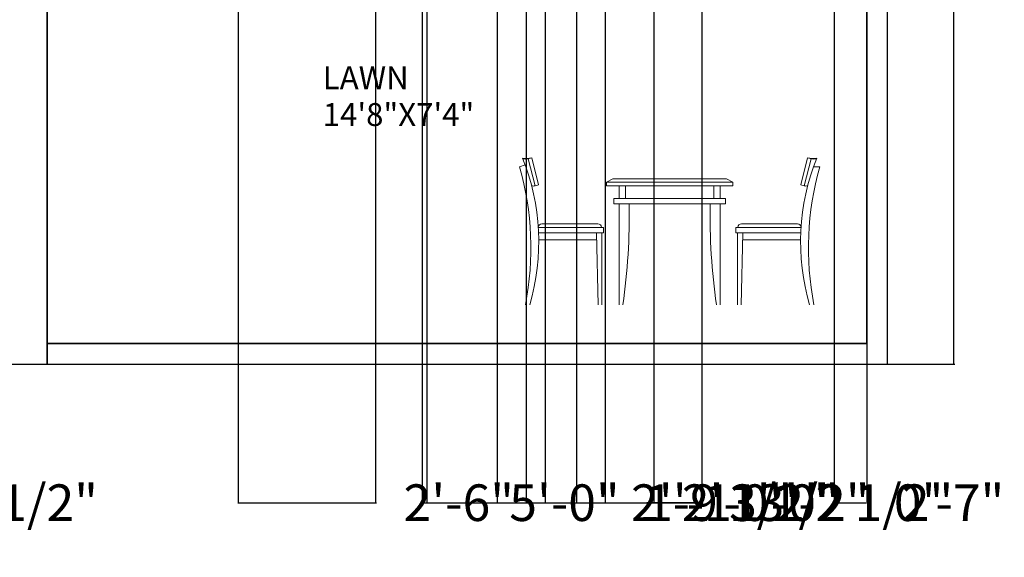
# Model space of a CAD drawing. Units: inches. Extents: x -26 to 385, y 12 to 697.
# Tile 2 of 13: x 136 to 351, y 12 to 130. Entities that reach past the tile are written whole.
import ezdxf

# ---------------------------------------------------------------- set-up
doc = ezdxf.new("R2010")
doc.units = ezdxf.units.IN
doc.header["$MEASUREMENT"] = 0
for name, color, linetype, lineweight in [('A-ANNO-DIMS', 4, 'Continuous', 18), ('A-AREA-IDEN', 4, 'Continuous', 18), ('A-WALL', 40, 'Continuous', 35), ('C-PROP', 40, 'Continuous', 25), ('Furniture', 210, 'Continuous', 15)]:
    doc.layers.add(name, color=color, linetype=linetype, lineweight=lineweight)
doc.styles.get("Standard").update_dxf_attribs({"font": 'italic8.shx'})
doc.dimstyles.get("Standard").update_dxf_attribs({"dimtxt": 8, "dimasz": 0.18, "dimexe": 0.18, "dimexo": 0.0625, "dimgap": 0.09, "dimtad": 0, "dimtih": 1, "dimtoh": 1, "dimdec": 4, "dimzin": 0, "dimdsep": 46, "dimlunit": 3, "dimtxsty": 'Standard', "dimcen": 0.09, "dimclrd": 2, "dimclre": 3, "dimclrt": 6, "dimadec": 0, "dimazin": 0, "dimtfac": 1, "dimtdec": 4, "dimtofl": 0, "dimtmove": 0, "dimatfit": 3, "dimfxl": 1, "dimtolj": 1, "dimtzin": 0, "dimarcsym": 0})

# ---------------------------------------------------------------- blocks, each defined once
blk = doc.blocks.new('*D2')
at = {"layer": 'A-ANNO-DIMS', "color": 0, "lineweight": -2, "transparency": 16777216}
for p, q in [((325.19, 654.38), (339.84, 654.38)), ((339.66, 654.2), (339.66, 359.23)), ((339.66, 54.56), (339.66, 349.53)), ((325.19, 54.38), (339.84, 54.38))]:
    blk.add_line(p, q, dxfattribs=at)
at = {"layer": 'A-ANNO-DIMS', "color": 0, "transparency": 16777216}
for points in [[(339.63, 654.2), (339.69, 654.2), (339.66, 654.38)], [(339.63, 54.56), (339.69, 54.56), (339.66, 54.38)]]:
    blk.add_solid(points, dxfattribs=at)
at = {"layer": 'Defpoints', "color": 0, "transparency": 16777216}
for p in [(325.13, 654.38), (325.13, 54.38), (339.66, 54.38)]:
    blk.add_point(p, dxfattribs=at)
at = {"layer": 'A-ANNO-DIMS', "color": 0, "transparency": 16777216, "insert": (339.66, 354.38), "char_height": 8, "attachment_point": 5}
blk.add_mtext("\\A1;50'", dxfattribs=at)
blk = doc.blocks.new('*D25')
at = {"layer": 'A-ANNO-DIMS', "color": 3, "lineweight": -2, "transparency": 16777216}
for p, q in [((284.629322, 368.316588), (284.629322, 23.949088)), ((320.629322, 368.316588), (320.629322, 23.949088))]:
    blk.add_line(p, q, dxfattribs=at)
at = {"layer": 'A-ANNO-DIMS', "color": 2, "lineweight": -2, "transparency": 16777216}
for p, q in [((284.449322, 24.129088), (284.269322, 24.129088)), ((320.809322, 24.129088), (320.989322, 24.129088))]:
    blk.add_line(p, q, dxfattribs=at)
at = {"layer": 'A-ANNO-DIMS', "color": 2, "transparency": 16777216}
for points in [[(284.449322, 24.159088), (284.449322, 24.099088), (284.629322, 24.129088)], [(320.809322, 24.159088), (320.809322, 24.099088), (320.629322, 24.129088)]]:
    blk.add_solid(points, dxfattribs=at)
at = {"layer": 'Defpoints', "color": 0, "transparency": 16777216}
for p in [(284.629322, 368.379088), (320.629322, 368.379088), (320.629322, 24.129088)]:
    blk.add_point(p, dxfattribs=at)
at = {"layer": 'A-ANNO-DIMS', "color": 6, "transparency": 16777216, "insert": (302.629322, 24.129088), "char_height": 8, "attachment_point": 5}
blk.add_mtext('\\A1;3\'-0"', dxfattribs=at)
blk = doc.blocks.new('*D31')
at = {"layer": 'A-ANNO-DIMS', "color": 3, "lineweight": -2, "transparency": 16777216}
for p, q in [((239.89, 166.08), (239.89, 23.95)), ((263.51, 166.08), (263.51, 23.95))]:
    blk.add_line(p, q, dxfattribs=at)
at = {"layer": 'A-ANNO-DIMS', "color": 2, "lineweight": -2, "transparency": 16777216}
for p, q in [((240.07, 24.13), (263.33, 24.13)), ((263.51, 24.13), (263.69, 24.13))]:
    blk.add_line(p, q, dxfattribs=at)
at = {"layer": 'A-ANNO-DIMS', "color": 2, "transparency": 16777216}
for points in [[(240.07, 24.16), (240.07, 24.1), (239.89, 24.13)], [(263.33, 24.16), (263.33, 24.1), (263.51, 24.13)]]:
    blk.add_solid(points, dxfattribs=at)
at = {"layer": 'Defpoints', "color": 0, "transparency": 16777216}
for p in [(239.89, 166.14), (263.51, 166.14), (263.51, 24.13)]:
    blk.add_point(p, dxfattribs=at)
at = {"layer": 'A-ANNO-DIMS', "color": 6, "transparency": 16777216, "insert": (296.73, 24.13), "char_height": 8, "attachment_point": 5}
blk.add_mtext('\\A1;1\'-11 1/2"', dxfattribs=at)
blk = doc.blocks.new('*D33')
at = {"layer": 'A-ANNO-DIMS', "color": 3, "lineweight": -2, "transparency": 16777216}
for p, q in [((58.47, 279.82), (58.47, 23.95)), ((97.85, 279.82), (97.85, 23.95))]:
    blk.add_line(p, q, dxfattribs=at)
at = {"layer": 'A-ANNO-DIMS', "color": 2, "lineweight": -2, "transparency": 16777216}
for p, q in [((58.65, 24.13), (97.67, 24.13)), ((97.85, 24.13), (98.03, 24.13))]:
    blk.add_line(p, q, dxfattribs=at)
at = {"layer": 'A-ANNO-DIMS', "color": 2, "transparency": 16777216}
for points in [[(58.65, 24.16), (58.65, 24.1), (58.47, 24.13)], [(97.67, 24.16), (97.67, 24.1), (97.85, 24.13)]]:
    blk.add_solid(points, dxfattribs=at)
at = {"layer": 'Defpoints', "color": 0, "transparency": 16777216}
for p in [(58.47, 279.88), (97.85, 279.88), (97.85, 24.13)]:
    blk.add_point(p, dxfattribs=at)
at = {"layer": 'A-ANNO-DIMS', "color": 6, "transparency": 16777216, "insert": (131.26, 24.13), "char_height": 8, "attachment_point": 5}
blk.add_mtext('\\A1;3\'-3 1/2"', dxfattribs=at)
blk = doc.blocks.new('*D37')
at = {"layer": 'A-ANNO-DIMS', "color": 3, "lineweight": -2, "transparency": 16777216}
for p, q in [((223.55, 597.32), (223.55, 23.95)), ((257.22, 597.32), (257.22, 23.95))]:
    blk.add_line(p, q, dxfattribs=at)
at = {"layer": 'A-ANNO-DIMS', "color": 2, "lineweight": -2, "transparency": 16777216}
for p, q in [((223.73, 24.13), (257.04, 24.13)), ((257.22, 24.13), (257.4, 24.13))]:
    blk.add_line(p, q, dxfattribs=at)
at = {"layer": 'A-ANNO-DIMS', "color": 2, "transparency": 16777216}
for points in [[(223.73, 24.16), (223.73, 24.1), (223.55, 24.13)], [(257.04, 24.16), (257.04, 24.1), (257.22, 24.13)]]:
    blk.add_solid(points, dxfattribs=at)
at = {"layer": 'Defpoints', "color": 0, "transparency": 16777216}
for p in [(223.55, 597.38), (257.22, 597.38), (257.22, 24.13)]:
    blk.add_point(p, dxfattribs=at)
at = {"layer": 'A-ANNO-DIMS', "color": 6, "transparency": 16777216, "insert": (290.63, 24.13), "char_height": 8, "attachment_point": 5}
blk.add_mtext('\\A1;2\'-9 1/2"', dxfattribs=at)
blk = doc.blocks.new('*D39')
at = {"layer": 'A-ANNO-DIMS', "color": 3, "lineweight": -2, "transparency": 16777216}
for p, q in [((183.36, 597.32), (183.36, 23.95)), ((213.36, 597.32), (213.36, 23.95))]:
    blk.add_line(p, q, dxfattribs=at)
at = {"layer": 'A-ANNO-DIMS', "color": 2, "lineweight": -2, "transparency": 16777216}
for p, q in [((183.54, 24.13), (213.18, 24.13)), ((213.36, 24.13), (213.54, 24.13))]:
    blk.add_line(p, q, dxfattribs=at)
at = {"layer": 'A-ANNO-DIMS', "color": 2, "transparency": 16777216}
for points in [[(183.54, 24.16), (183.54, 24.1), (183.36, 24.13)], [(213.18, 24.16), (213.18, 24.1), (213.36, 24.13)]]:
    blk.add_solid(points, dxfattribs=at)
at = {"layer": 'Defpoints', "color": 0, "transparency": 16777216}
for p in [(183.36, 597.38), (213.36, 597.38), (213.36, 24.13)]:
    blk.add_point(p, dxfattribs=at)
at = {"layer": 'A-ANNO-DIMS', "color": 6, "transparency": 16777216, "insert": (231.53, 24.13), "char_height": 8, "attachment_point": 5}
blk.add_mtext('\\A1;2\'-6"', dxfattribs=at)
blk = doc.blocks.new('*D42')
at = {"layer": 'A-ANNO-DIMS', "color": 3, "lineweight": -2, "transparency": 16777216}
for p, q in [((250.37, 518.99), (250.37, 23.95)), ((274.13, 518.99), (274.13, 23.95))]:
    blk.add_line(p, q, dxfattribs=at)
at = {"layer": 'A-ANNO-DIMS', "color": 2, "lineweight": -2, "transparency": 16777216}
for p, q in [((250.55, 24.13), (273.95, 24.13)), ((274.13, 24.13), (274.31, 24.13))]:
    blk.add_line(p, q, dxfattribs=at)
at = {"layer": 'A-ANNO-DIMS', "color": 2, "transparency": 16777216}
for points in [[(250.55, 24.16), (250.55, 24.1), (250.37, 24.13)], [(273.95, 24.16), (273.95, 24.1), (274.13, 24.13)]]:
    blk.add_solid(points, dxfattribs=at)
at = {"layer": 'Defpoints', "color": 0, "transparency": 16777216}
for p in [(250.37, 519.05), (274.13, 519.05), (274.13, 24.13)]:
    blk.add_point(p, dxfattribs=at)
at = {"layer": 'A-ANNO-DIMS', "color": 6, "transparency": 16777216, "insert": (292.3, 24.13), "char_height": 8, "attachment_point": 5}
blk.add_mtext('\\A1;2\'-0"', dxfattribs=at)
blk = doc.blocks.new('*D46')
at = {"layer": 'A-ANNO-DIMS', "color": 3, "lineweight": -2, "transparency": 16777216}
for p, q in [((224.59, 477.32), (224.59, 23.95)), ((284.63, 477.32), (284.63, 23.95))]:
    blk.add_line(p, q, dxfattribs=at)
at = {"layer": 'A-ANNO-DIMS', "color": 2, "lineweight": -2, "transparency": 16777216}
for p, q in [((224.77, 24.13), (236.62, 24.13)), ((284.45, 24.13), (272.61, 24.13))]:
    blk.add_line(p, q, dxfattribs=at)
at = {"layer": 'A-ANNO-DIMS', "color": 2, "transparency": 16777216}
for points in [[(224.77, 24.16), (224.77, 24.1), (224.59, 24.13)], [(284.45, 24.16), (284.45, 24.1), (284.63, 24.13)]]:
    blk.add_solid(points, dxfattribs=at)
at = {"layer": 'Defpoints', "color": 0, "transparency": 16777216}
for p in [(224.59, 477.38), (284.63, 477.38), (284.63, 24.13)]:
    blk.add_point(p, dxfattribs=at)
at = {"layer": 'A-ANNO-DIMS', "color": 6, "transparency": 16777216, "insert": (254.61, 24.13), "char_height": 8, "attachment_point": 5}
blk.add_mtext('\\A1;5\'-0"', dxfattribs=at)
blk = doc.blocks.new('*D50')
at = {"layer": 'A-ANNO-DIMS', "color": 3, "lineweight": -2, "transparency": 16777216}
for p, q in [((246.28, 401.87), (246.28, 23.95)), ((284.63, 398.32), (284.63, 23.95))]:
    blk.add_line(p, q, dxfattribs=at)
at = {"layer": 'A-ANNO-DIMS', "color": 2, "lineweight": -2, "transparency": 16777216}
for p, q in [((246.46, 24.13), (284.45, 24.13)), ((284.63, 24.13), (284.81, 24.13))]:
    blk.add_line(p, q, dxfattribs=at)
at = {"layer": 'A-ANNO-DIMS', "color": 2, "transparency": 16777216}
for points in [[(246.46, 24.16), (246.46, 24.1), (246.28, 24.13)], [(284.45, 24.16), (284.45, 24.1), (284.63, 24.13)]]:
    blk.add_solid(points, dxfattribs=at)
at = {"layer": 'Defpoints', "color": 0, "transparency": 16777216}
for p in [(246.28, 401.93), (284.63, 398.38), (284.63, 24.13)]:
    blk.add_point(p, dxfattribs=at)
at = {"layer": 'A-ANNO-DIMS', "color": 6, "transparency": 16777216, "insert": (318.04, 24.13), "char_height": 8, "attachment_point": 5}
blk.add_mtext('\\A1;3\'-2 1/2"', dxfattribs=at)
blk = doc.blocks.new('*D52')
at = {"layer": 'A-ANNO-DIMS', "color": 3, "lineweight": -2, "transparency": 16777216}
for p, q in [((313.49, 154.68), (313.49, 23.95)), ((320.63, 147.82), (320.63, 23.95))]:
    blk.add_line(p, q, dxfattribs=at)
at = {"layer": 'A-ANNO-DIMS', "color": 2, "lineweight": -2, "transparency": 16777216}
for p, q in [((313.67, 24.13), (320.45, 24.13)), ((320.63, 24.13), (320.81, 24.13))]:
    blk.add_line(p, q, dxfattribs=at)
at = {"layer": 'A-ANNO-DIMS', "color": 2, "transparency": 16777216}
for points in [[(313.67, 24.16), (313.67, 24.1), (313.49, 24.13)], [(320.45, 24.16), (320.45, 24.1), (320.63, 24.13)]]:
    blk.add_solid(points, dxfattribs=at)
at = {"layer": 'Defpoints', "color": 0, "transparency": 16777216}
for p in [(313.49, 154.74), (320.63, 147.88), (320.63, 24.13)]:
    blk.add_point(p, dxfattribs=at)
at = {"layer": 'A-ANNO-DIMS', "color": 6, "transparency": 16777216, "insert": (338.61, 24.13), "char_height": 8, "attachment_point": 5}
blk.add_mtext('\\A1;0\'-7"', dxfattribs=at)

msp = doc.modelspace()

# ---------------------------------------------------------------- linework, layer by layer
at = {"layer": 'A-WALL'}
for p, q in [((141.62932, 158.90341), (141.62932, 54.37909)), ((320.62932, 58.87909), (320.62932, 143.37909)), ((141.62932, 58.87909), (320.62932, 58.87909))]:
    msp.add_line(p, q, dxfattribs=at)
at = {"layer": 'C-PROP'}
for p, q in [((325.12932, 54.37909), (325.12932, 654.37909)), ((25.12932, 54.37909), (325.12932, 54.37909))]:
    msp.add_line(p, q, dxfattribs=at)
at = {"layer": 'Furniture'}
for p, q in [((246.71323, 99.26482), (247.44895, 99.45015)), ((246.71323, 99.26482), (248.20083, 93.35932)), ((247.47678, 99.45716), (248.96614, 93.54465)), ((307.69739, 99.45716), (306.20803, 93.54465)), ((308.46094, 99.26482), (306.97334, 93.35932)), ((308.46094, 99.26482), (307.72522, 99.45015)), ((244.77299, 97.49513), (246.02022, 97.95115)), ((308.98976, 97.49513), (310.40118, 97.49513)), ((263.80758, 94.11927), (265.18553, 94.90667)), ((265.18553, 94.90667), (289.98863, 94.90667)), ((289.98863, 94.90667), (291.36658, 94.11927)), ((248.23042, 93.35932), (248.96614, 93.54465)), ((263.80758, 94.11927), (291.36658, 94.11927)), ((263.80758, 94.11927), (263.80758, 93.33187)), ((263.80758, 93.33187), (291.36658, 93.33187)), ((266.56348, 93.33187), (266.56348, 90.57597)), ((267.93107, 90.57597), (267.93107, 93.33187)), ((287.2431, 90.57597), (287.2431, 93.33187)), ((288.61068, 93.33187), (288.61068, 90.57597)), ((291.36658, 94.11927), (291.36658, 93.33187)), ((306.94375, 93.35932), (306.20803, 93.54465)), ((265.38238, 90.57597), (289.79178, 90.57597)), ((265.38238, 90.57597), (265.38238, 89.39487)), ((289.79178, 90.57597), (289.79178, 89.39487)), ((265.38238, 89.39487), (289.79178, 89.39487)), ((266.56348, 89.39487), (266.56348, 67.34767)), ((288.61068, 89.39487), (288.61068, 67.34767)), ((263.17002, 84.27677), (248.89939, 84.27677)), ((261.8895, 85.06417), (249.68679, 85.06417)), ((263.17002, 83.09567), (263.17002, 84.27677)), ((292.00415, 84.27677), (306.27478, 84.27677)), ((292.00415, 83.09567), (292.00415, 84.27677)), ((293.28467, 85.06417), (305.48738, 85.06417)), ((263.17002, 83.09567), (248.9614, 83.09567)), ((261.59522, 83.09567), (261.98892, 67.34767)), ((262.77632, 83.09567), (262.77632, 67.34767)), ((292.00415, 83.09567), (306.21277, 83.09567)), ((292.39785, 83.09567), (292.39785, 67.34767)), ((293.57895, 83.09567), (293.18525, 67.34767)), ((261.63459, 81.52087), (248.9614, 81.52087)), ((293.53958, 81.52087), (306.21277, 81.52087))]:
    msp.add_line(p, q, dxfattribs=at)
for centre, radius, start, end in [((246.388, 104.13383), 4.80234, 258.798532, 282.7633354), ((199.9756, 81.11607), 49.02578, 343.6896616, 21.9263097), ((246.11583, 102.1925), 2.98801, 258.467063, 281.532937), ((355.19857, 81.11607), 49.02578, 158.0736903, 196.3103384), ((308.78617, 104.13383), 4.80234, 257.2366646, 281.201468), ((309.05833, 102.1925), 2.98801, 258.467063, 281.532937), ((183.49115, 79.76125), 63.7962, 348.7797098, 16.1395142), ((371.68302, 79.76125), 63.7962, 163.8604858, 191.2202902), ((247.81306, 94.79624), 1.49555, 256.0176019, 285.0974231), ((307.3611, 94.79624), 1.49555, 254.9025769, 283.9823981), ((136.57655, 86.52563), 132.17307, 351.6570855, 1.2438872), ((418.59762, 86.52563), 132.17307, 178.7561128, 188.3429145), ((249.68679, 84.27677), 0.7874, 90, 180), ((261.8895, 84.27677), 0.7874, 0, 90), ((293.28467, 84.27677), 0.7874, 90, 180), ((305.48738, 84.27677), 0.7874, 0, 90)]:
    msp.add_arc(centre, radius, start, end, dxfattribs=at)

# ---------------------------------------------------------------- texts
at = {"layer": 'A-AREA-IDEN'}
for s, p in [('LAWN', (201.82242, 114.44952)), ('14\'8"X7\'4"', (201.82242, 106.41746))]:
    msp.add_text(s, height=5, dxfattribs=at).set_placement(p)

# ---------------------------------------------------------------- dimensions: what is measured, and where the dimension line sits
at = {"layer": 'A-ANNO-DIMS'}
dim = msp.add_linear_dim(base=(339.65968, 54.37909), p1=(325.12932, 654.37909), p2=(325.12932, 54.37909), angle=90, dimstyle='Standard', override={"dimclrd": 0, "dimclre": 0, "dimclrt": 0}, dxfattribs=at)
dim.commit()
dim.dimension.update_dxf_attribs({"geometry": '*D2', "text_midpoint": (339.65968, 354.37909)})
for base, p1, p2, picture, middle in [((213.35855, 24.12909), (183.35855, 597.37909), (213.35855, 597.37909), '*D39', (231.53331, 24.12909)), ((257.21981, 24.12909), (223.54856, 597.37909), (257.21981, 597.37909), '*D37', (290.63267, 24.12909)), ((274.12932, 24.12909), (250.37102, 519.05498), (274.12932, 519.05498), '*D42', (292.30408, 24.12909)), ((284.62932, 24.12909), (224.59493, 477.37909), (284.62932, 477.37909), '*D46', (254.61213, 24.12909)), ((284.62932, 24.12909), (246.27828, 401.934), (284.62932, 398.37909), '*D50', (318.04218, 24.12909)), ((320.62932, 24.12909), (284.62932, 368.37909), (320.62932, 368.37909), '*D25', (302.62932, 24.12909)), ((97.84659, 24.12909), (58.46784, 279.87909), (97.84659, 279.87909), '*D33', (131.25945, 24.12909)), ((263.50956, 24.12909), (239.88756, 166.14113), (263.50956, 166.14113), '*D31', (296.73194, 24.12909)), ((320.62932, 24.12909), (313.48771, 154.73754), (320.62932, 147.87909), '*D52', (338.61361, 24.12909))]:
    dim = msp.add_linear_dim(base=base, p1=p1, p2=p2, dimstyle='Standard', override={"dimdec": 1, "dimlfac": 1, "dimrnd": 0, "dimzin": 1, "dimdsep": 46, "dimlunit": 4, "dimfrac": 2}, dxfattribs=at)
    dim.commit()
    dim.dimension.update_dxf_attribs({"geometry": picture, "text_midpoint": middle})

doc.saveas('drawing.dxf')
